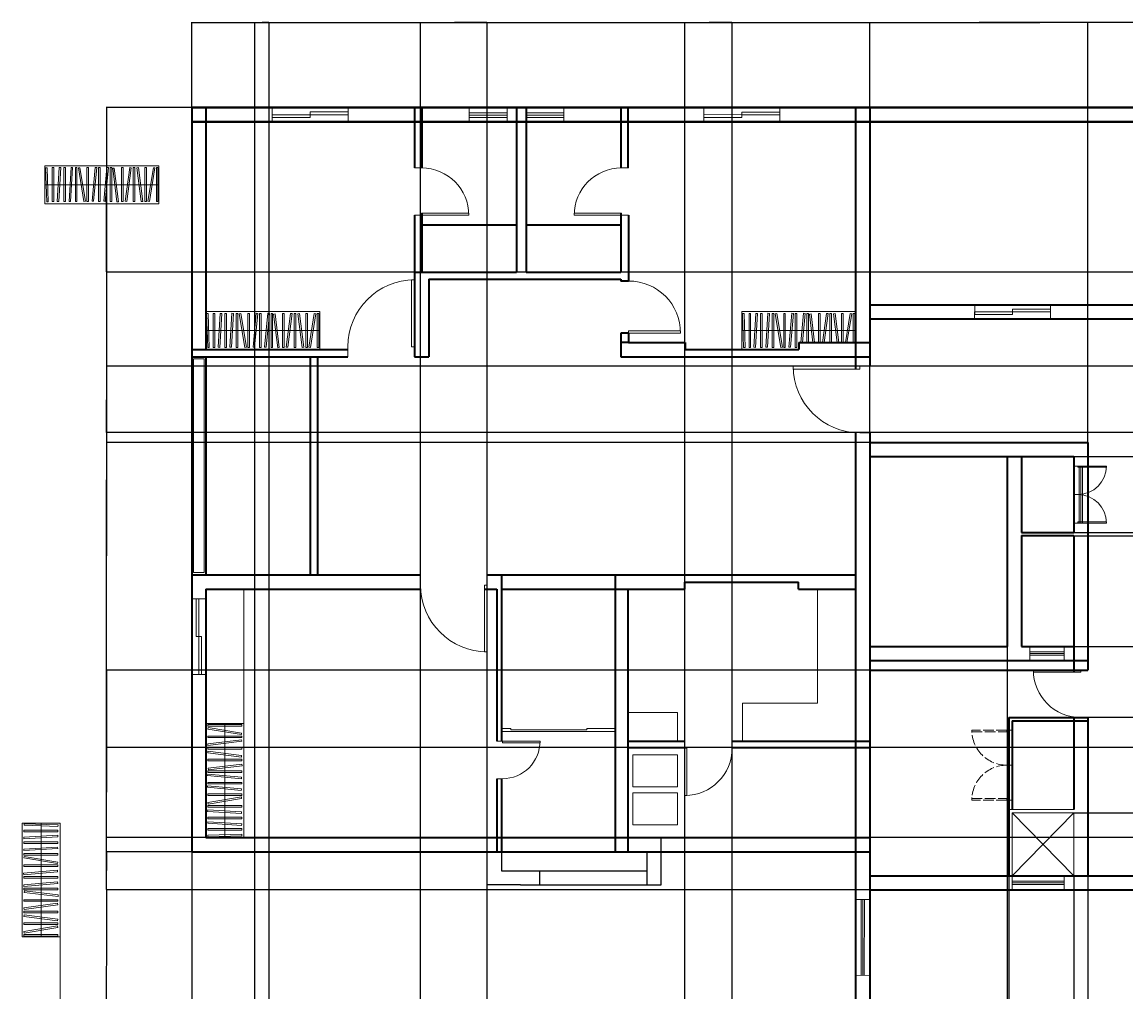
# Model space of a CAD drawing. Units: inches. Extents: x 531915 to 533151, y 849859 to 851471.
# Tile 5 of 7: x 531915 to 532614, y 850858 to 851471. Entities that reach past the tile are written whole.
import ezdxf

# ---------------------------------------------------------------- set-up
doc = ezdxf.new("R2010")
doc.units = ezdxf.units.IN
doc.linetypes.add('ACAD_ISO02W100', pattern=[15, 12, -3])
for name, color, linetype, lineweight in [('A-ANNO-DIMS', 2, 'Continuous', 18), ('A-DOOR', 3, 'Continuous', 18), ('A-DOOR-HIDN', 3, 'ACAD_ISO02W100', 18), ('A-FLOR-CASE', 9, 'Continuous', 18), ('A-FLOR-FIXT', 8, 'Continuous', 18), ('A-FLOR-HRAL', 4, 'Continuous', 20), ('A-FLOR-SHFT', 9, 'Continuous', 18), ('A-FLOR-SLAB', 7, 'Continuous', 25), ('A-FURN', 8, 'Continuous', 13), ('A-GLAZ', 4, 'Continuous', 18), ('A-WALL', 7, 'Continuous', 35)]:
    doc.layers.add(name, color=color, linetype=linetype, lineweight=lineweight)
doc.styles.get("Standard").update_dxf_attribs({"font": 'arial.ttf'})
doc.dimstyles.get("Standard").update_dxf_attribs({"dimtxt": 0.18, "dimasz": 0.18, "dimexe": 0.18, "dimexo": 0.0625, "dimgap": 0.09, "dimtad": 0, "dimtih": 1, "dimtoh": 1, "dimdec": 4, "dimzin": 0, "dimdsep": 46, "dimtxsty": 'Standard', "dimcen": 0.09, "dimadec": 0, "dimazin": 0, "dimtfac": 1, "dimtdec": 4, "dimtofl": 0, "dimtmove": 0, "dimatfit": 3, "dimfxl": 1, "dimtolj": 1, "dimtzin": 0, "dimarcsym": 0})

# ---------------------------------------------------------------- blocks, each defined once
blk = doc.blocks.new('*U2')
for p, q in [((0, 0), (0, -6)), ((40, 0), (40, -6))]:
    blk.add_line(p, q)
blk.add_lwpolyline([(0, 0), (0, 40), (1.75, 40), (1.75, 0)], close=True)
blk.add_arc((0, 0), 40, 0, 90)
blk = doc.blocks.new('WARDROBE-72')
blk.add_line((12, 0), (12, 72))
for points in [[(24, 0), (24, 72), (0, 72), (0, 0)], [(1.15, 70.47), (1.15, 71.48), (22.64, 71.48), (22.64, 70.47)], [(1.15, 63.15), (1.15, 64.16), (22.64, 64.16), (22.64, 63.15)], [(1.21, 68.56), (1.37, 69.55), (22.58, 66.07), (22.41, 65.07)], [(1.15, 55.83), (1.15, 56.84), (22.64, 56.84), (22.64, 55.83)], [(1.3, 58.13), (1.17, 59.13), (22.48, 61.86), (22.61, 60.86)], [(1.11, 53.59), (1.24, 54.59), (22.54, 51.79), (22.41, 50.79)], [(1.15, 48.51), (1.15, 49.52), (22.64, 49.52), (22.64, 48.51)], [(1.15, 41.19), (1.15, 42.2), (22.64, 42.2), (22.64, 41.19)], [(1.55, 42.84), (1.42, 43.84), (22.76, 46.42), (22.88, 45.42)], [(1.04, 39.13), (1.13, 40.14), (22.52, 38.16), (22.43, 37.15)], [(0.98, 31.76), (1.07, 32.76), (22.47, 30.78), (22.37, 29.78)], [(1.15, 33.87), (1.15, 34.88), (22.64, 34.88), (22.64, 33.87)], [(1.15, 26.55), (1.15, 27.56), (22.64, 27.56), (22.64, 26.55)], [(1.38, 21.1), (1.21, 22.1), (22.4, 25.68), (22.57, 24.68)], [(1.05, 16.46), (1.11, 17.47), (22.56, 16.21), (22.5, 15.2)], [(1.15, 19.23), (1.15, 20.24), (22.64, 20.24), (22.64, 19.23)], [(1.11, 8.97), (1.17, 9.98), (22.62, 8.71), (22.56, 7.7)], [(1.15, 11.91), (1.15, 12.92), (22.64, 12.92), (22.64, 11.91)], [(1.15, 4.59), (1.15, 5.6), (22.64, 5.6), (22.64, 4.59)], [(1.25, 0.42), (1.22, 1.43), (22.7, 2.11), (22.73, 1.1)]]:
    blk.add_lwpolyline(points, close=True)
blk = doc.blocks.new('WARDROBE-72-RECESSED')
blk.add_line((0, 12), (72, 12))
for points in [[(72, 0), (72, 24), (0, 24), (0, 0), (36.16, 0)], [(37.42, 4.5), (39.13, 22.96), (40.14, 22.87), (38.44, 4.5)], [(41.19, 4.5), (41.19, 22.85), (42.2, 22.85), (42.2, 4.5)], [(45.01, 4.5), (42.84, 22.45), (43.84, 22.58), (46.03, 4.5)], [(48.51, 4.5), (48.51, 22.85), (49.52, 22.85), (49.52, 4.5)], [(51.17, 4.5), (53.59, 22.89), (54.59, 22.76), (52.19, 4.5)], [(55.83, 4.5), (55.83, 22.85), (56.84, 22.85), (56.84, 4.5)], [(60.46, 4.5), (58.13, 22.7), (59.13, 22.83), (61.48, 4.5)], [(63.15, 4.5), (63.15, 22.85), (64.16, 22.85), (64.16, 4.5)], [(65.55, 4.5), (68.56, 22.79), (69.55, 22.63), (66.57, 4.5)], [(70.47, 4.5), (70.47, 22.85), (71.48, 22.85), (71.48, 4.5)]]:
    blk.add_lwpolyline(points)
for points in [[(0.42, 22.75), (1.43, 22.78), (2.11, 1.3), (1.1, 1.27)], [(4.59, 22.85), (5.6, 22.85), (5.6, 1.36), (4.59, 1.36)], [(8.97, 22.89), (9.98, 22.83), (8.71, 1.38), (7.7, 1.44)], [(11.91, 22.85), (12.92, 22.85), (12.92, 1.36), (11.91, 1.36)], [(16.46, 22.95), (17.47, 22.89), (16.21, 1.44), (15.2, 1.5)], [(19.23, 22.85), (20.24, 22.85), (20.24, 1.36), (19.23, 1.36)], [(21.1, 22.62), (22.1, 22.79), (25.68, 1.6), (24.68, 1.43)], [(26.55, 22.85), (27.56, 22.85), (27.56, 1.36), (26.55, 1.36)], [(31.76, 23.02), (32.76, 22.93), (30.78, 1.53), (29.78, 1.63)], [(33.87, 22.85), (34.88, 22.85), (34.88, 1.36), (33.87, 1.36)]]:
    blk.add_lwpolyline(points, close=True)
blk = doc.blocks.new('WINDOW-SLIDING-48')
for p, q in [((0, 9), (0, 0)), ((48, 9), (48, 0)), ((0, 4.5), (48, 4.5))]:
    blk.add_line(p, q)
for points in [[(24, 4.5), (0, 4.5), (0, 2.84), (24, 2.84)], [(24, 4.5), (48, 4.5), (48, 6.29), (24, 6.29)]]:
    blk.add_lwpolyline(points, close=True)
blk = doc.blocks.new('WINDOW-VENT-24')
blk.add_line((0, 1.44), (24, 1.44))
blk.add_lwpolyline([(0, 2.89), (24, 2.89), (24, 0), (0, 0)], close=True)
blk = doc.blocks.new('UTILITY-FIXTURES-PAIR')
for points in [[(0, 24.11), (28.12, 24.11), (28.12, 44.31), (0, 44.31)], [(0, 0), (28.12, 0), (28.12, 20.2), (0, 20.2)]]:
    blk.add_lwpolyline(points, close=True)
blk = doc.blocks.new('SLIDING-PANEL-72')
for p, q in [((0, 2), (6, 2)), ((6, 2), (6, 1)), ((6, 1), (54, 1)), ((54, 2), (72, 2)), ((54, 2), (54, 1)), ((0, 0), (72, 0))]:
    blk.add_line(p, q)
blk = doc.blocks.new('COUNTER-L-RETURN')
for p, q in [((47.51, 96), (47.51, 24)), ((0, 24), (47.51, 24)), ((0, 24), (0, 0))]:
    blk.add_line(p, q)
blk = doc.blocks.new('COUNTER-END-RETURN')
for p in [(0, 18), (31.29, 0)]:
    blk.add_line(p, (31.29, 18))
blk = doc.blocks.new('*D37')
at = {"layer": 'A-ANNO-DIMS', "color": 0, "lineweight": -2, "transparency": 16777216}
for p, q in [((532022.8, 851416.94), (532022.8, 851470.96)), ((532022.98, 851470.78), (532559.45, 851470.78)), ((533096.62, 851470.78), (532560.15, 851470.78)), ((533096.8, 851416.94), (533096.8, 851470.96))]:
    blk.add_line(p, q, dxfattribs=at)
at = {"layer": 'A-ANNO-DIMS', "color": 0, "transparency": 16777216}
for points in [[(532022.98, 851470.81), (532022.98, 851470.75), (532022.8, 851470.78)], [(533096.62, 851470.81), (533096.62, 851470.75), (533096.8, 851470.78)]]:
    blk.add_solid(points, dxfattribs=at)
at = {"layer": 'Defpoints', "color": 0, "transparency": 16777216}
for p in [(533096.8, 851470.78), (532022.8, 851416.87), (533096.8, 851416.87)]:
    blk.add_point(p, dxfattribs=at)
at = {"layer": 'A-ANNO-DIMS', "color": 0, "transparency": 16777216, "insert": (532559.8, 851470.78), "char_height": 0.18, "attachment_point": 5}
blk.add_mtext('\\A1;1074', dxfattribs=at)
blk = doc.blocks.new('*D39')
at = {"layer": 'A-ANNO-DIMS', "color": 0, "lineweight": -2, "transparency": 16777216}
for p, q in [((532022.74, 851416.87), (531968.71, 851416.87)), ((531968.89, 851416.69), (531968.89, 851181.81)), ((531968.89, 850946.55), (531968.89, 851181.44)), ((532022.74, 850946.37), (531968.71, 850946.37))]:
    blk.add_line(p, q, dxfattribs=at)
at = {"layer": 'A-ANNO-DIMS', "color": 0, "transparency": 16777216}
for points in [[(531968.86, 851416.69), (531968.92, 851416.69), (531968.89, 851416.87)], [(531968.86, 850946.55), (531968.92, 850946.55), (531968.89, 850946.37)]]:
    blk.add_solid(points, dxfattribs=at)
at = {"layer": 'Defpoints', "color": 0, "transparency": 16777216}
for p in [(532022.8, 851416.87), (531968.89, 850946.37), (532022.8, 850946.37)]:
    blk.add_point(p, dxfattribs=at)
at = {"layer": 'A-ANNO-DIMS', "color": 0, "transparency": 16777216, "insert": (531968.89, 851181.62), "char_height": 0.18, "attachment_point": 5}
blk.add_mtext('\\A1;470.5', dxfattribs=at)
blk = doc.blocks.new('*D40')
at = {"layer": 'A-ANNO-DIMS', "color": 0, "lineweight": -2, "transparency": 16777216}
for p, q in [((532022.74, 850946.37), (531968.71, 850946.37)), ((531968.89, 850946.19), (531968.89, 850934.48)), ((531968.89, 850922.41), (531968.89, 850934.12)), ((532451.74, 850922.23), (531968.71, 850922.23))]:
    blk.add_line(p, q, dxfattribs=at)
at = {"layer": 'A-ANNO-DIMS', "color": 0, "transparency": 16777216}
for points in [[(531968.86, 850946.19), (531968.92, 850946.19), (531968.89, 850946.37)], [(531968.86, 850922.41), (531968.92, 850922.41), (531968.89, 850922.23)]]:
    blk.add_solid(points, dxfattribs=at)
at = {"layer": 'Defpoints', "color": 0, "transparency": 16777216}
for p in [(532022.8, 850946.37), (531968.89, 850922.23), (532451.8, 850922.23)]:
    blk.add_point(p, dxfattribs=at)
at = {"layer": 'A-ANNO-DIMS', "color": 0, "transparency": 16777216, "insert": (531968.89, 850934.3), "char_height": 0.18, "attachment_point": 5}
blk.add_mtext('\\A1;24.14', dxfattribs=at)
blk = doc.blocks.new('*D41')
at = {"layer": 'A-ANNO-DIMS', "color": 0, "lineweight": -2, "transparency": 16777216}
for p, q in [((532451.74, 850922.23), (531968.71, 850922.23)), ((531968.89, 850922.05), (531968.89, 850874.49)), ((531968.89, 850826.55), (531968.89, 850874.12)), ((532062.74, 850826.37), (531968.71, 850826.37))]:
    blk.add_line(p, q, dxfattribs=at)
at = {"layer": 'A-ANNO-DIMS', "color": 0, "transparency": 16777216}
for points in [[(531968.86, 850922.05), (531968.92, 850922.05), (531968.89, 850922.23)], [(531968.86, 850826.55), (531968.92, 850826.55), (531968.89, 850826.37)]]:
    blk.add_solid(points, dxfattribs=at)
at = {"layer": 'Defpoints', "color": 0, "transparency": 16777216}
for p in [(532451.8, 850922.23), (531968.89, 850826.37), (532062.8, 850826.37)]:
    blk.add_point(p, dxfattribs=at)
at = {"layer": 'A-ANNO-DIMS', "color": 0, "transparency": 16777216, "insert": (531968.89, 850874.3), "char_height": 0.18, "attachment_point": 5}
blk.add_mtext('\\A1;95.86', dxfattribs=at)
blk = doc.blocks.new('*D46')
at = {"layer": 'A-ANNO-DIMS', "color": 0, "lineweight": -2, "transparency": 16777216}
for p, q in [((532022.8, 850946.31), (532022.8, 850315.34)), ((532062.8, 850826.31), (532062.8, 850315.34)), ((532022.98, 850315.52), (532042.58, 850315.52)), ((532062.62, 850315.52), (532043.03, 850315.52))]:
    blk.add_line(p, q, dxfattribs=at)
at = {"layer": 'A-ANNO-DIMS', "color": 0, "transparency": 16777216}
for points in [[(532022.98, 850315.55), (532022.98, 850315.49), (532022.8, 850315.52)], [(532062.62, 850315.55), (532062.62, 850315.49), (532062.8, 850315.52)]]:
    blk.add_solid(points, dxfattribs=at)
at = {"layer": 'Defpoints', "color": 0, "transparency": 16777216}
for p in [(532022.8, 850946.37), (532062.8, 850826.37), (532062.8, 850315.52)]:
    blk.add_point(p, dxfattribs=at)
at = {"layer": 'A-ANNO-DIMS', "color": 0, "transparency": 16777216, "insert": (532042.8, 850315.52), "char_height": 0.18, "attachment_point": 5}
blk.add_mtext('\\A1;40', dxfattribs=at)
blk = doc.blocks.new('*D59')
at = {"layer": 'A-ANNO-DIMS', "color": 0, "lineweight": -2, "transparency": 16777216}
for p, q in [((533087.74, 851012.37), (531968.71, 851012.37)), ((531968.89, 851012.19), (531968.89, 850984.06)), ((531968.89, 850955.55), (531968.89, 850983.69)), ((533087.74, 850955.37), (531968.71, 850955.37))]:
    blk.add_line(p, q, dxfattribs=at)
at = {"layer": 'A-ANNO-DIMS', "color": 0, "transparency": 16777216}
for points in [[(531968.86, 851012.19), (531968.92, 851012.19), (531968.89, 851012.37)], [(531968.86, 850955.55), (531968.92, 850955.55), (531968.89, 850955.37)]]:
    blk.add_solid(points, dxfattribs=at)
at = {"layer": 'Defpoints', "color": 0, "transparency": 16777216}
for p in [(533087.8, 851012.37), (531968.89, 850955.37), (533087.8, 850955.37)]:
    blk.add_point(p, dxfattribs=at)
at = {"layer": 'A-ANNO-DIMS', "color": 0, "transparency": 16777216, "insert": (531968.89, 850983.87), "char_height": 0.18, "attachment_point": 5}
blk.add_mtext('\\A1;57', dxfattribs=at)
blk = doc.blocks.new('*D68')
at = {"layer": 'A-ANNO-DIMS', "color": 0, "lineweight": -2, "transparency": 16777216}
for p, q in [((532451.74, 851205.23), (531968.71, 851205.23)), ((531968.89, 851205.05), (531968.89, 851133.41)), ((531968.89, 851061.41), (531968.89, 851133.05)), ((532451.74, 851061.23), (531968.71, 851061.23))]:
    blk.add_line(p, q, dxfattribs=at)
at = {"layer": 'A-ANNO-DIMS', "color": 0, "transparency": 16777216}
for points in [[(531968.86, 851205.05), (531968.92, 851205.05), (531968.89, 851205.23)], [(531968.86, 851061.41), (531968.92, 851061.41), (531968.89, 851061.23)]]:
    blk.add_solid(points, dxfattribs=at)
at = {"layer": 'Defpoints', "color": 0, "transparency": 16777216}
for p in [(532451.8, 851205.23), (531968.89, 851061.23), (532451.8, 851061.23)]:
    blk.add_point(p, dxfattribs=at)
at = {"layer": 'A-ANNO-DIMS', "color": 0, "transparency": 16777216, "insert": (531968.89, 851133.23), "char_height": 0.18, "attachment_point": 5}
blk.add_mtext('\\A1;144', dxfattribs=at)
blk = doc.blocks.new('*D69')
at = {"layer": 'A-ANNO-DIMS', "color": 0, "lineweight": -2, "transparency": 16777216}
for p, q in [((532451.74, 851061.23), (531968.71, 851061.23)), ((531968.89, 851061.05), (531968.89, 850991.92)), ((531968.89, 850922.41), (531968.89, 850991.55)), ((532451.74, 850922.23), (531968.71, 850922.23))]:
    blk.add_line(p, q, dxfattribs=at)
at = {"layer": 'A-ANNO-DIMS', "color": 0, "transparency": 16777216}
for points in [[(531968.86, 851061.05), (531968.92, 851061.05), (531968.89, 851061.23)], [(531968.86, 850922.41), (531968.92, 850922.41), (531968.89, 850922.23)]]:
    blk.add_solid(points, dxfattribs=at)
at = {"layer": 'Defpoints', "color": 0, "transparency": 16777216}
for p in [(532451.8, 851061.23), (531968.89, 850922.23), (532451.8, 850922.23)]:
    blk.add_point(p, dxfattribs=at)
at = {"layer": 'A-ANNO-DIMS', "color": 0, "transparency": 16777216, "insert": (531968.89, 850991.73), "char_height": 0.18, "attachment_point": 5}
blk.add_mtext('\\A1;139', dxfattribs=at)
blk = doc.blocks.new('*D70')
at = {"layer": 'A-ANNO-DIMS', "color": 0, "lineweight": -2, "transparency": 16777216}
for p, q in [((532451.8, 851205.3), (532451.8, 851470.96)), ((532451.98, 851470.78), (532520.52, 851470.78)), ((532589.62, 851470.78), (532521.09, 851470.78)), ((532589.8, 851205.3), (532589.8, 851470.96))]:
    blk.add_line(p, q, dxfattribs=at)
at = {"layer": 'A-ANNO-DIMS', "color": 0, "transparency": 16777216}
for points in [[(532451.98, 851470.81), (532451.98, 851470.75), (532451.8, 851470.78)], [(532589.62, 851470.81), (532589.62, 851470.75), (532589.8, 851470.78)]]:
    blk.add_solid(points, dxfattribs=at)
at = {"layer": 'Defpoints', "color": 0, "transparency": 16777216}
for p in [(532589.8, 851470.78), (532451.8, 851205.23), (532589.8, 851205.23)]:
    blk.add_point(p, dxfattribs=at)
at = {"layer": 'A-ANNO-DIMS', "color": 0, "transparency": 16777216, "insert": (532520.8, 851470.78), "char_height": 0.18, "attachment_point": 5}
blk.add_mtext('\\A1;138', dxfattribs=at)
blk = doc.blocks.new('*D71')
at = {"layer": 'A-ANNO-DIMS', "color": 0, "lineweight": -2, "transparency": 16777216}
for p, q in [((532589.8, 850931.17), (532589.8, 850315.34)), ((532667.8, 850931.17), (532667.8, 850315.34)), ((532589.98, 850315.52), (532628.59, 850315.52)), ((532667.62, 850315.52), (532629.02, 850315.52))]:
    blk.add_line(p, q, dxfattribs=at)
at = {"layer": 'A-ANNO-DIMS', "color": 0, "transparency": 16777216}
for points in [[(532589.98, 850315.55), (532589.98, 850315.49), (532589.8, 850315.52)], [(532667.62, 850315.55), (532667.62, 850315.49), (532667.8, 850315.52)]]:
    blk.add_solid(points, dxfattribs=at)
at = {"layer": 'Defpoints', "color": 0, "transparency": 16777216}
for p in [(532589.8, 850931.23), (532667.8, 850931.23), (532667.8, 850315.52)]:
    blk.add_point(p, dxfattribs=at)
at = {"layer": 'A-ANNO-DIMS', "color": 0, "transparency": 16777216, "insert": (532628.8, 850315.52), "char_height": 0.18, "attachment_point": 5}
blk.add_mtext('\\A1;78', dxfattribs=at)
blk = doc.blocks.new('*D72')
at = {"layer": 'A-ANNO-DIMS', "color": 0, "lineweight": -2, "transparency": 16777216}
for p, q in [((532451.8, 850931.17), (532451.8, 850315.34)), ((532539.8, 850931.17), (532539.8, 850315.34)), ((532451.98, 850315.52), (532495.59, 850315.52)), ((532539.62, 850315.52), (532496.02, 850315.52))]:
    blk.add_line(p, q, dxfattribs=at)
at = {"layer": 'A-ANNO-DIMS', "color": 0, "transparency": 16777216}
for points in [[(532451.98, 850315.55), (532451.98, 850315.49), (532451.8, 850315.52)], [(532539.62, 850315.55), (532539.62, 850315.49), (532539.8, 850315.52)]]:
    blk.add_solid(points, dxfattribs=at)
at = {"layer": 'Defpoints', "color": 0, "transparency": 16777216}
for p in [(532451.8, 850931.23), (532539.8, 850931.23), (532539.8, 850315.52)]:
    blk.add_point(p, dxfattribs=at)
at = {"layer": 'A-ANNO-DIMS', "color": 0, "transparency": 16777216, "insert": (532495.8, 850315.52), "char_height": 0.18, "attachment_point": 5}
blk.add_mtext('\\A1;88', dxfattribs=at)
blk = doc.blocks.new('*D73')
at = {"layer": 'A-ANNO-DIMS', "color": 0, "lineweight": -2, "transparency": 16777216}
for p, q in [((532539.8, 850931.17), (532539.8, 850315.34)), ((532580.8, 850931.17), (532580.8, 850315.34)), ((532539.98, 850315.52), (532560.1, 850315.52)), ((532580.62, 850315.52), (532560.51, 850315.52))]:
    blk.add_line(p, q, dxfattribs=at)
at = {"layer": 'A-ANNO-DIMS', "color": 0, "transparency": 16777216}
for points in [[(532539.98, 850315.55), (532539.98, 850315.49), (532539.8, 850315.52)], [(532580.62, 850315.55), (532580.62, 850315.49), (532580.8, 850315.52)]]:
    blk.add_solid(points, dxfattribs=at)
at = {"layer": 'Defpoints', "color": 0, "transparency": 16777216}
for p in [(532539.8, 850931.23), (532580.8, 850931.23), (532580.8, 850315.52)]:
    blk.add_point(p, dxfattribs=at)
at = {"layer": 'A-ANNO-DIMS', "color": 0, "transparency": 16777216, "insert": (532560.3, 850315.52), "char_height": 0.18, "attachment_point": 5}
blk.add_mtext('\\A1;41', dxfattribs=at)
blk = doc.blocks.new('*D74')
at = {"layer": 'A-ANNO-DIMS', "color": 0, "lineweight": -2, "transparency": 16777216}
for p, q in [((532580.87, 850971.01), (533150.9, 850971.01)), ((533150.72, 850970.83), (533150.72, 850951.31)), ((533150.72, 850931.41), (533150.72, 850950.94)), ((532580.87, 850931.23), (533150.9, 850931.23))]:
    blk.add_line(p, q, dxfattribs=at)
at = {"layer": 'A-ANNO-DIMS', "color": 0, "transparency": 16777216}
for points in [[(533150.69, 850970.83), (533150.75, 850970.83), (533150.72, 850971.01)], [(533150.69, 850931.41), (533150.75, 850931.41), (533150.72, 850931.23)]]:
    blk.add_solid(points, dxfattribs=at)
at = {"layer": 'Defpoints', "color": 0, "transparency": 16777216}
for p in [(532580.8, 850971.01), (533150.72, 850971.01), (532580.8, 850931.23)]:
    blk.add_point(p, dxfattribs=at)
at = {"layer": 'A-ANNO-DIMS', "color": 0, "transparency": 16777216, "insert": (533150.72, 850951.12), "char_height": 0.18, "attachment_point": 5}
blk.add_mtext('\\A1;39.78', dxfattribs=at)
blk = doc.blocks.new('*D75')
at = {"layer": 'A-ANNO-DIMS', "color": 0, "lineweight": -2, "transparency": 16777216}
for p, q in [((532580.87, 851031.56), (533150.9, 851031.56)), ((533150.72, 851031.38), (533150.72, 851001.47)), ((533150.72, 850971.19), (533150.72, 851001.11)), ((532580.87, 850971.01), (533150.9, 850971.01))]:
    blk.add_line(p, q, dxfattribs=at)
at = {"layer": 'A-ANNO-DIMS', "color": 0, "transparency": 16777216}
for points in [[(533150.69, 851031.38), (533150.75, 851031.38), (533150.72, 851031.56)], [(533150.69, 850971.19), (533150.75, 850971.19), (533150.72, 850971.01)]]:
    blk.add_solid(points, dxfattribs=at)
at = {"layer": 'Defpoints', "color": 0, "transparency": 16777216}
for p in [(532580.8, 851031.56), (533150.72, 851031.56), (532580.8, 850971.01)]:
    blk.add_point(p, dxfattribs=at)
at = {"layer": 'A-ANNO-DIMS', "color": 0, "transparency": 16777216, "insert": (533150.72, 851001.29), "char_height": 0.18, "attachment_point": 5}
blk.add_mtext('\\A1;60.55', dxfattribs=at)
blk = doc.blocks.new('*D76')
at = {"layer": 'A-ANNO-DIMS', "color": 0, "lineweight": -2, "transparency": 16777216}
for p, q in [((532820.74, 851416.87), (531968.71, 851416.87)), ((531968.89, 851416.69), (531968.89, 851365.03)), ((531968.89, 851313), (531968.89, 851364.67)), ((532825.24, 851312.82), (531968.71, 851312.82))]:
    blk.add_line(p, q, dxfattribs=at)
at = {"layer": 'A-ANNO-DIMS', "color": 0, "transparency": 16777216}
for points in [[(531968.86, 851416.69), (531968.92, 851416.69), (531968.89, 851416.87)], [(531968.86, 851313), (531968.92, 851313), (531968.89, 851312.82)]]:
    blk.add_solid(points, dxfattribs=at)
at = {"layer": 'Defpoints', "color": 0, "transparency": 16777216}
for p in [(532820.8, 851416.87), (531968.89, 851312.82), (532825.3, 851312.82)]:
    blk.add_point(p, dxfattribs=at)
at = {"layer": 'A-ANNO-DIMS', "color": 0, "transparency": 16777216, "insert": (531968.89, 851364.85), "char_height": 0.18, "attachment_point": 5}
blk.add_mtext('\\A1;104.05', dxfattribs=at)
blk = doc.blocks.new('*D78')
at = {"layer": 'A-ANNO-DIMS', "color": 0, "lineweight": -2, "transparency": 16777216}
for p, q in [((532451.8, 851196.17), (532451.8, 850315.34)), ((532538.8, 851196.17), (532538.8, 850315.34)), ((532451.98, 850315.52), (532495.09, 850315.52)), ((532538.62, 850315.52), (532495.52, 850315.52))]:
    blk.add_line(p, q, dxfattribs=at)
at = {"layer": 'A-ANNO-DIMS', "color": 0, "transparency": 16777216}
for points in [[(532451.98, 850315.55), (532451.98, 850315.49), (532451.8, 850315.52)], [(532538.62, 850315.55), (532538.62, 850315.49), (532538.8, 850315.52)]]:
    blk.add_solid(points, dxfattribs=at)
at = {"layer": 'Defpoints', "color": 0, "transparency": 16777216}
for p in [(532451.8, 851196.23), (532538.8, 851196.23), (532538.8, 850315.52)]:
    blk.add_point(p, dxfattribs=at)
at = {"layer": 'A-ANNO-DIMS', "color": 0, "transparency": 16777216, "insert": (532495.3, 850315.52), "char_height": 0.18, "attachment_point": 5}
blk.add_mtext('\\A1;87', dxfattribs=at)
blk = doc.blocks.new('*D79')
at = {"layer": 'A-ANNO-DIMS', "color": 0, "lineweight": -2, "transparency": 16777216}
for p, q in [((532580.87, 851196.23), (533150.9, 851196.23)), ((533150.72, 851196.05), (533150.72, 851172.42)), ((533150.72, 851148.41), (533150.72, 851172.05)), ((532580.87, 851148.23), (533150.9, 851148.23))]:
    blk.add_line(p, q, dxfattribs=at)
at = {"layer": 'A-ANNO-DIMS', "color": 0, "transparency": 16777216}
for points in [[(533150.69, 851196.05), (533150.75, 851196.05), (533150.72, 851196.23)], [(533150.69, 851148.41), (533150.75, 851148.41), (533150.72, 851148.23)]]:
    blk.add_solid(points, dxfattribs=at)
at = {"layer": 'Defpoints', "color": 0, "transparency": 16777216}
for p in [(532580.8, 851196.23), (532580.8, 851148.23), (533150.72, 851148.23)]:
    blk.add_point(p, dxfattribs=at)
at = {"layer": 'A-ANNO-DIMS', "color": 0, "transparency": 16777216, "insert": (533150.72, 851172.23), "char_height": 0.18, "attachment_point": 5}
blk.add_mtext('\\A1;48', dxfattribs=at)
blk = doc.blocks.new('*D80')
at = {"layer": 'A-ANNO-DIMS', "color": 0, "lineweight": -2, "transparency": 16777216}
for p, q in [((532580.87, 851146.23), (533150.9, 851146.23)), ((533150.72, 851146.05), (533150.72, 851111.42)), ((533150.72, 851076.41), (533150.72, 851111.05)), ((532580.87, 851076.23), (533150.9, 851076.23))]:
    blk.add_line(p, q, dxfattribs=at)
at = {"layer": 'A-ANNO-DIMS', "color": 0, "transparency": 16777216}
for points in [[(533150.69, 851146.05), (533150.75, 851146.05), (533150.72, 851146.23)], [(533150.69, 851076.41), (533150.75, 851076.41), (533150.72, 851076.23)]]:
    blk.add_solid(points, dxfattribs=at)
at = {"layer": 'Defpoints', "color": 0, "transparency": 16777216}
for p in [(532580.8, 851146.23), (532580.8, 851076.23), (533150.72, 851076.23)]:
    blk.add_point(p, dxfattribs=at)
at = {"layer": 'A-ANNO-DIMS', "color": 0, "transparency": 16777216, "insert": (533150.72, 851111.23), "char_height": 0.18, "attachment_point": 5}
blk.add_mtext('\\A1;70', dxfattribs=at)
blk = doc.blocks.new('*D81')
at = {"layer": 'A-ANNO-DIMS', "color": 0, "lineweight": -2, "transparency": 16777216}
for p, q in [((532062.8, 850826.44), (532062.8, 851470.96)), ((532062.98, 851470.78), (532067.16, 851470.78)), ((532071.62, 851470.78), (532067.45, 851470.78)), ((532071.8, 850817.44), (532071.8, 851470.96))]:
    blk.add_line(p, q, dxfattribs=at)
at = {"layer": 'A-ANNO-DIMS', "color": 0, "transparency": 16777216}
for points in [[(532062.98, 851470.81), (532062.98, 851470.75), (532062.8, 851470.78)], [(532071.62, 851470.81), (532071.62, 851470.75), (532071.8, 851470.78)]]:
    blk.add_solid(points, dxfattribs=at)
at = {"layer": 'Defpoints', "color": 0, "transparency": 16777216}
for p in [(532071.8, 851470.78), (532062.8, 850826.37), (532071.8, 850817.37)]:
    blk.add_point(p, dxfattribs=at)
at = {"layer": 'A-ANNO-DIMS', "color": 0, "transparency": 16777216, "insert": (532067.3, 851470.78), "char_height": 0.18, "attachment_point": 5}
blk.add_mtext('\\A1;9', dxfattribs=at)
blk = doc.blocks.new('*D83')
at = {"layer": 'A-ANNO-DIMS', "color": 0, "lineweight": -2, "transparency": 16777216}
for p, q in [((532667.74, 851253.37), (531968.71, 851253.37)), ((531968.89, 851253.19), (531968.89, 851232.55)), ((531968.89, 851211.55), (531968.89, 851232.19)), ((532667.74, 851211.37), (531968.71, 851211.37))]:
    blk.add_line(p, q, dxfattribs=at)
at = {"layer": 'A-ANNO-DIMS', "color": 0, "transparency": 16777216}
for points in [[(531968.86, 851253.19), (531968.92, 851253.19), (531968.89, 851253.37)], [(531968.86, 851211.55), (531968.92, 851211.55), (531968.89, 851211.37)]]:
    blk.add_solid(points, dxfattribs=at)
at = {"layer": 'Defpoints', "color": 0, "transparency": 16777216}
for p in [(531968.89, 851253.37), (532667.8, 851253.37), (532667.8, 851211.37)]:
    blk.add_point(p, dxfattribs=at)
at = {"layer": 'A-ANNO-DIMS', "color": 0, "transparency": 16777216, "insert": (531968.89, 851232.37), "char_height": 0.18, "attachment_point": 5}
blk.add_mtext('\\A1;42', dxfattribs=at)
blk = doc.blocks.new('*D85')
at = {"layer": 'A-ANNO-DIMS', "color": 0, "lineweight": -2, "transparency": 16777216}
for p, q in [((532334.8, 850439.44), (532334.8, 851470.96)), ((532334.98, 851470.78), (532349.32, 851470.78)), ((532364.58, 851470.78), (532350.25, 851470.78)), ((532364.76, 850439.44), (532364.76, 851470.96))]:
    blk.add_line(p, q, dxfattribs=at)
at = {"layer": 'A-ANNO-DIMS', "color": 0, "transparency": 16777216}
for points in [[(532334.98, 851470.81), (532334.98, 851470.75), (532334.8, 851470.78)], [(532364.58, 851470.81), (532364.58, 851470.75), (532364.76, 851470.78)]]:
    blk.add_solid(points, dxfattribs=at)
at = {"layer": 'Defpoints', "color": 0, "transparency": 16777216}
for p in [(532364.76, 851470.78), (532334.8, 850439.37), (532364.76, 850439.37)]:
    blk.add_point(p, dxfattribs=at)
at = {"layer": 'A-ANNO-DIMS', "color": 0, "transparency": 16777216, "insert": (532349.78, 851470.78), "char_height": 0.18, "attachment_point": 5}
blk.add_mtext('\\A1;29.954', dxfattribs=at)
blk = doc.blocks.new('*D86')
at = {"layer": 'A-ANNO-DIMS', "color": 0, "lineweight": -2, "transparency": 16777216}
for p, q in [((532167.55, 850544.44), (532167.55, 851470.96)), ((532167.73, 851470.78), (532188.28, 851470.78)), ((532209.62, 851470.78), (532189.08, 851470.78)), ((532209.8, 850544.44), (532209.8, 851470.96))]:
    blk.add_line(p, q, dxfattribs=at)
at = {"layer": 'A-ANNO-DIMS', "color": 0, "transparency": 16777216}
for points in [[(532167.73, 851470.81), (532167.73, 851470.75), (532167.55, 851470.78)], [(532209.62, 851470.81), (532209.62, 851470.75), (532209.8, 851470.78)]]:
    blk.add_solid(points, dxfattribs=at)
at = {"layer": 'Defpoints', "color": 0, "transparency": 16777216}
for p in [(532209.8, 851470.78), (532167.55, 850544.37), (532209.8, 850544.37)]:
    blk.add_point(p, dxfattribs=at)
at = {"layer": 'A-ANNO-DIMS', "color": 0, "transparency": 16777216, "insert": (532188.68, 851470.78), "char_height": 0.18, "attachment_point": 5}
blk.add_mtext('\\A1;42.25', dxfattribs=at)

msp = doc.modelspace()

# ---------------------------------------------------------------- linework, layer by layer
at = {"layer": 'A-DOOR'}
for p, q in [((532580.8048, 851190.2344), (532589.8048, 851190.2344)), ((532584.3048, 851190.2344), (532584.3048, 851154.2344)), ((532585.3048, 851190.2344), (532585.3048, 851154.2344)), ((532586.3048, 851190.2344), (532586.3048, 851154.2344)), ((532580.8048, 851154.2344), (532589.8048, 851154.2344))]:
    msp.add_line(p, q, dxfattribs=at)
at = {"layer": 'A-FLOR-CASE'}
msp.add_line((532442.8048, 851112.374), (532418.8048, 851112.374), dxfattribs=at)
at = {"layer": 'A-FLOR-HRAL'}
msp.add_lwpolyline([(532023.9094, 851258.0527), (532030.6325, 851258.0527), (532030.6325, 851122.9414), (532023.9094, 851122.9414)], close=True, dxfattribs=at)
at = {"layer": 'A-FLOR-SHFT'}
for p, q in [((532539.8048, 850973.0147), (532580.8048, 850973.0147)), ((532541.8048, 850971.0147), (532580.8048, 850971.0147)), ((532541.8048, 850931.2344), (532580.8048, 850971.0147)), ((532541.8048, 850971.0147), (532580.8048, 850931.2344)), ((532541.8048, 850971.0147), (532541.8048, 850931.2344)), ((532580.8048, 850971.0147), (532580.8048, 850931.2344))]:
    msp.add_line(p, q, dxfattribs=at)
at = {"layer": 'A-FLOR-SLAB'}
for p, q in [((532319.8048, 850925.374), (532319.8048, 850955.374)), ((532209.8048, 850925.374), (532209.8048, 850946.374)), ((532218.8048, 850946.374), (532218.8048, 850934.374)), ((532310.8048, 850946.374), (532310.8048, 850925.374)), ((532218.8048, 850934.374), (532230.8048, 850934.374)), ((532218.8048, 850934.374), (532242.8048, 850934.374)), ((532230.8048, 850934.374), (532310.8048, 850934.374)), ((532242.8048, 850934.374), (532242.8048, 850925.374)), ((532230.8048, 850925.374), (532209.8048, 850925.374)), ((532230.8048, 850925.374), (532310.8048, 850925.374)), ((532310.8048, 850925.374), (532319.8048, 850925.374))]:
    msp.add_line(p, q, dxfattribs=at)
at = {"layer": 'A-FURN'}
for p, q in [((532055.8048, 851027.374), (532055.8048, 851112.374)), ((531939.4832, 850892.5471), (531939.4832, 850807.5471))]:
    msp.add_line(p, q, dxfattribs=at)
at = {"layer": 'A-GLAZ'}
for p, q in [((532198.3048, 851416.874), (532198.3048, 851407.874)), ((532222.3048, 851416.874), (532222.3048, 851407.874)), ((532258.3048, 851416.874), (532258.3048, 851407.874)), ((532022.8048, 851106.374), (532031.8048, 851106.374)), ((532553.1172, 851076.2344), (532553.1172, 851067.2344)), ((532553.1172, 851072.7344), (532574.8048, 851072.7344)), ((532553.1172, 851071.7344), (532574.8048, 851071.7344)), ((532574.8048, 851076.2344), (532574.8048, 851067.2344)), ((532553.1172, 851070.7344), (532574.8048, 851070.7344)), ((532541.8048, 850931.2344), (532541.8048, 850922.2344)), ((532574.8048, 850931.2344), (532574.8048, 850922.2344)), ((532541.8048, 850927.7344), (532574.8048, 850927.7344)), ((532541.8048, 850926.7344), (532574.8048, 850926.7344)), ((532541.8048, 850925.7344), (532574.8048, 850925.7344)), ((532442.8817, 850916.1195), (532451.8817, 850916.2349)), ((532446.3817, 850916.1788), (532446.3048, 850868.1868)), ((532447.3817, 850916.1772), (532447.3048, 850868.1852)), ((532448.3817, 850916.1756), (532448.3048, 850868.1836)), ((532442.8048, 850868.1234), (532451.8048, 850868.247))]:
    msp.add_line(p, q, dxfattribs=at)
at = {"layer": 'A-WALL'}
for p, q in [((532022.8048, 851416.874), (533096.8048, 851416.874)), ((532022.8048, 851416.874), (532022.8048, 850946.374)), ((532022.8048, 851416.874), (532022.8048, 850946.374)), ((533096.8048, 851416.874), (532022.8048, 851416.874)), ((532031.8048, 851416.874), (532031.8048, 851263.874)), ((532031.8048, 851416.874), (532163.8048, 851416.874)), ((532163.8048, 851416.874), (532163.8048, 851378.7079)), ((532168.3048, 851416.874), (532168.3048, 851378.7079)), ((532228.3048, 851416.874), (532228.3048, 851312.8243)), ((532234.3048, 851416.874), (532234.3048, 851312.8243)), ((532294.3048, 851416.874), (532294.3048, 851378.706)), ((532298.8048, 851416.874), (532298.8048, 851378.7079)), ((532298.8048, 851416.874), (532442.8048, 851416.874)), ((532442.8048, 851416.874), (532442.8048, 851251.5304)), ((532451.8048, 851416.874), (532451.8048, 851253.374)), ((532451.8048, 851416.874), (532667.8048, 851416.874)), ((532667.8048, 851416.874), (532451.8048, 851416.874)), ((532022.8048, 851407.874), (533096.8048, 851407.874)), ((533096.8048, 851407.874), (532022.8048, 851407.874)), ((532163.8048, 851348.8243), (532163.8048, 851259.374)), ((532168.3048, 851350.1317), (532168.3048, 851312.8243)), ((532294.3048, 851350.1317), (532294.3048, 851312.8243)), ((532299.125, 851348.8243), (532299.125, 851307.227)), ((532168.3048, 851342.8243), (532228.3048, 851342.8243)), ((532234.3048, 851342.8243), (532294.3048, 851342.8243)), ((532163.8048, 851312.8243), (532228.3048, 851312.8243)), ((532234.3048, 851312.8243), (532294.3048, 851312.8243)), ((532172.8048, 851308.3243), (532172.8048, 851259.374)), ((532172.8048, 851308.3243), (532294.3048, 851308.3243)), ((532294.3048, 851308.3243), (532294.3048, 851307.227)), ((532299.125, 851307.2354), (532294.3048, 851307.2354)), ((532451.8048, 851292.2344), (532667.8048, 851292.2344)), ((532451.8048, 851283.2344), (532667.8048, 851283.2344)), ((532299.125, 851274.374), (532294.3048, 851274.374)), ((532294.3048, 851274.374), (532294.3048, 851259.374)), ((532299.125, 851274.374), (532299.125, 851268.374)), ((532299.125, 851268.374), (532294.3048, 851268.374)), ((532299.125, 851268.374), (532334.9649, 851268.374)), ((532299.125, 851268.374), (532334.9649, 851268.374)), ((532299.125, 851268.374), (532334.9649, 851268.374)), ((532334.9649, 851268.374), (532334.9649, 851263.874)), ((532406.9649, 851268.374), (532406.9649, 851263.874)), ((532406.9649, 851268.374), (532442.8048, 851268.374)), ((532406.9649, 851268.374), (532442.8048, 851268.374)), ((532406.9649, 851268.374), (532451.8048, 851268.374)), ((532022.8048, 851263.874), (532121.553, 851263.874)), ((532334.9649, 851263.874), (532406.9649, 851263.874)), ((532022.8048, 851259.374), (532121.553, 851259.374)), ((532031.8048, 851259.374), (532031.8048, 851121.374)), ((532097.8048, 851259.374), (532097.8048, 851121.374)), ((532102.3048, 851259.374), (532102.3048, 851121.374)), ((532163.8048, 851259.374), (532172.8048, 851259.374)), ((532294.3048, 851259.374), (532451.8048, 851259.374)), ((532442.8048, 851211.3197), (532442.8048, 850946.374)), ((532451.8048, 851211.2344), (532451.8048, 850946.374)), ((532451.8048, 851211.2344), (532451.8048, 851205.2344)), ((532451.8048, 851205.2344), (532589.8048, 851205.2344)), ((532589.8048, 851205.2344), (532589.8048, 851061.2344)), ((532451.8048, 851196.2344), (532580.8048, 851196.2344)), ((532538.8048, 851196.2344), (532538.8048, 851076.2344)), ((532547.8048, 851196.2344), (532547.8048, 851148.2344)), ((532580.8048, 851196.2344), (532580.8048, 851148.2344)), ((532547.8048, 851148.2344), (532580.8048, 851148.2344)), ((532547.8048, 851146.2344), (532580.8048, 851146.2344)), ((532547.8048, 851146.2344), (532547.8048, 851076.2344)), ((532580.8048, 851146.2344), (532580.8048, 851076.2344)), ((532022.8048, 851121.374), (532167.8048, 851121.374)), ((532209.8048, 851121.374), (532442.8048, 851121.374)), ((532218.8048, 851121.374), (532218.8048, 851016.374)), ((532290.8048, 851121.374), (532290.8048, 850946.374)), ((532334.8048, 851116.874), (532406.8048, 851116.874)), ((532334.8048, 851112.374), (532334.8048, 851116.874)), ((532406.8048, 851112.374), (532406.8048, 851116.874)), ((532031.8048, 851112.374), (532167.8048, 851112.374)), ((532031.8048, 851112.374), (532031.8048, 850955.374)), ((532207.9563, 851112.374), (532215.8048, 851112.374)), ((532215.8048, 851112.374), (532215.8048, 851016.374)), ((532218.8048, 851112.374), (532334.8048, 851112.374)), ((532298.8048, 851112.374), (532298.8048, 850946.374)), ((532298.8048, 851112.374), (532334.8048, 851112.374)), ((532406.8048, 851112.374), (532442.8048, 851112.374)), ((532406.8048, 851112.374), (532442.8048, 851112.374)), ((532451.8048, 851076.2344), (532538.8048, 851076.2344)), ((532547.8048, 851076.2344), (532580.8048, 851076.2344)), ((532580.8048, 851076.2344), (532580.8048, 851067.2344)), ((532451.8048, 851067.2344), (532589.8048, 851067.2344)), ((532580.8048, 851067.2344), (532580.8048, 851059.9215)), ((532451.8048, 851061.2344), (532589.8048, 851061.2344)), ((532539.8048, 851031.2344), (532589.8048, 851031.2344)), ((532539.8048, 851031.2344), (532539.8048, 851023.2344)), ((532541.8048, 851029.2344), (532541.8048, 851023.2344)), ((532541.8048, 851029.2344), (532589.8048, 851029.2344)), ((532580.8048, 851031.5642), (532580.8048, 850973.0147)), ((532589.8048, 851031.2344), (532589.8048, 850931.2344)), ((532539.8048, 851023.2344), (532539.8048, 850979.0147)), ((532541.8048, 851023.2344), (532541.8048, 850979.0147)), ((532298.8048, 851016.374), (532334.8048, 851016.374)), ((532364.7592, 851016.374), (532451.8048, 851016.374)), ((532298.8048, 851012.374), (532334.8048, 851012.374)), ((532364.7592, 851012.374), (532451.8048, 851012.374)), ((532215.8048, 850992.5523), (532215.8048, 850946.374)), ((532218.8048, 850992.5523), (532218.8048, 850946.374)), ((532539.8048, 850979.0147), (532539.8048, 850931.2344)), ((532541.8048, 850979.0147), (532541.8048, 850973.0147)), ((532031.8048, 850955.374), (532451.8048, 850955.374)), ((532022.8048, 850946.374), (532451.8048, 850946.374)), ((532442.8048, 850946.374), (532442.8048, 850922.119)), ((532442.8048, 850946.374), (532442.8048, 850826.374)), ((532451.8048, 850946.374), (532451.8048, 850931.2344)), ((532442.8048, 850931.2344), (532442.8048, 850369.374)), ((532451.8048, 850931.2344), (532667.8048, 850931.2344)), ((532451.8048, 850931.2344), (532451.8048, 850369.374)), ((532451.8048, 850922.2344), (532667.8048, 850922.2344))]:
    msp.add_line(p, q, dxfattribs=at)

# ---------------------------------------------------------------- block references
at = {"layer": 'A-DOOR'}
for p, xscale, yscale, zscale, rotation in [((532168.2873, 851348.8243), -0.7470890379753774, 0.7470890379753774, 0.7470890379753774, 270), ((532294.6424, 851348.8243), 0.7470890379753774, 0.7470890379753774, 0.7470890379753774, 90.00000000000003), ((532299.2327, 851274.374), -0.8213266256042635, 0.8213266256042635, 0.8213266256042635, 270), ((532445.4838, 851253.374), -1.053488616942954, 1.053488616942954, 1.053488616942954, 90), ((532583.5048, 851190.2344), 0.4499999999970897, 0.4499999999970897, 0.4499999999970897, 270), ((532583.5048, 851154.2344), -0.4499999999970897, 0.4499999999970897, 0.4499999999970897, 270), ((532209.8048, 851115.0362), 1.056294156906435, 1.056294156906435, 1.056294156906435, 180), ((532585.3034, 851061.2344), -0.7502326097997817, 0.7502326097997817, 0.7502326097997817, 90), ((532219.378, 851016.374), 0.5955413682082586, 0.5955413682082586, 0.5955413682082586, 270), ((532334.8048, 851011.8808), -0.7488601199280389, 0.7488601199280389, 0.7488601199280389, 180)]:
    msp.add_blockref('*U2', p, dxfattribs=dict(at, xscale=xscale, yscale=yscale, zscale=zscale, rotation=rotation))
at = {"layer": 'A-DOOR', "xscale": -1.056294156906435, "yscale": 1.056294156906435, "zscale": 1.056294156906435}
msp.add_blockref('*U2', (532163.8048, 851265.7117), dxfattribs=at)
at = {"layer": 'A-DOOR-HIDN', "yscale": 0.552746356571741, "zscale": 0.552746356571741}
for p, xscale, rotation in [((532538.4883, 851023.2344), -0.552746356571741, 90), ((532538.4883, 850979.0147), 0.552746356571741, 90.00000000000003)]:
    msp.add_blockref('*U2', p, dxfattribs=dict(at, xscale=xscale, rotation=rotation))
at = {"layer": 'A-FLOR-CASE'}
for name, p in [('COUNTER-L-RETURN', (532371.2933, 851016.374)), ('COUNTER-END-RETURN', (532298.8048, 851016.374))]:
    msp.add_blockref(name, p, dxfattribs=at)
at = {"layer": 'A-FLOR-FIXT'}
msp.add_blockref('UTILITY-FIXTURES-PAIR', (532301.9813, 850963.385), dxfattribs=at)
at = {"layer": 'A-FURN'}
for p, rotation in [((531929.9781, 851380.0997), 270.0000000012567), ((532031.8048, 851287.874), 269.9999999994314)]:
    msp.add_blockref('WARDROBE-72', p, dxfattribs=dict(at, rotation=rotation))
for name, p in [('WARDROBE-72-RECESSED', (532370.8048, 851263.874)), ('WARDROBE-72', (532031.8048, 850955.374))]:
    msp.add_blockref(name, p, dxfattribs=at)
at = {"layer": 'A-FURN', "extrusion": (0, 0, -1), "zscale": -1, "rotation": 180}
msp.add_blockref('WARDROBE-72', (-531915.4832, 850964.5471), dxfattribs=at)
at = {"layer": 'A-GLAZ'}
for name, p in [('WINDOW-SLIDING-48', (532073.8048, 851407.874)), ('WINDOW-VENT-24', (532198.3048, 851410.6579)), ('WINDOW-VENT-24', (532234.3048, 851410.6579)), ('SLIDING-PANEL-72', (532218.8048, 851022.374))]:
    msp.add_blockref(name, p, dxfattribs=at)
for p, rotation in [((532394.8104, 851416.875), 179.9286429434092), ((532566.1739, 851292.2355), 179.9286429431333), ((532022.8037, 851106.3796), 269.9286429430327)]:
    msp.add_blockref('WINDOW-SLIDING-48', p, dxfattribs=dict(at, rotation=rotation))

# ---------------------------------------------------------------- dimensions: what is measured, and where the dimension line sits
at = {"layer": 'A-ANNO-DIMS'}
for base, p1, p2, override, picture, middle in [((533096.8048, 851470.7848), (532022.8048, 851416.874), (533096.8048, 851416.874), {"dimdec": 0, "dimlfac": 1, "dimrnd": 0, "dimzin": 0, "dimdsep": 46, "dimlunit": 2}, '*D37', (532559.8048, 851470.7848)), ((532071.8048, 851470.7848), (532062.8048, 850826.374), (532071.8048, 850817.374), {"dimdec": 0, "dimlfac": 1, "dimrnd": 0, "dimzin": 0, "dimdsep": 46, "dimlunit": 2}, '*D81', (532067.3048, 851470.7848)), ((532209.8048, 851470.7848), (532167.553, 850544.374), (532209.8048, 850544.374), {"dimdec": 2, "dimlfac": 1, "dimrnd": 0, "dimzin": 0, "dimdsep": 46, "dimlunit": 2}, '*D86', (532188.6789, 851470.7848)), ((532364.7592, 851470.7848), (532334.8048, 850439.374), (532364.7592, 850439.374), {"dimdec": 3, "dimlfac": 1, "dimrnd": 0, "dimzin": 0, "dimdsep": 46, "dimlunit": 2}, '*D85', (532349.782, 851470.7848)), ((532589.8048, 851470.7848), (532451.8048, 851205.2344), (532589.8048, 851205.2344), {"dimdec": 0, "dimlfac": 1, "dimrnd": 0, "dimzin": 0, "dimdsep": 46, "dimlunit": 2}, '*D70', (532520.8048, 851470.7848)), ((532538.8048, 850315.524), (532451.8048, 851196.2344), (532538.8048, 851196.2344), {"dimdec": 0, "dimlfac": 1, "dimrnd": 0, "dimzin": 0, "dimdsep": 46, "dimlunit": 2}, '*D78', (532495.3048, 850315.524)), ((532062.8048, 850315.524), (532022.8048, 850946.374), (532062.8048, 850826.374), {"dimdec": 0, "dimlfac": 1, "dimrnd": 0, "dimzin": 0, "dimdsep": 46, "dimlunit": 2}, '*D46', (532042.8048, 850315.524)), ((532539.8048, 850315.524), (532451.8048, 850931.2344), (532539.8048, 850931.2344), {"dimdec": 0, "dimlfac": 1, "dimrnd": 0, "dimzin": 0, "dimdsep": 46, "dimlunit": 2}, '*D72', (532495.8048, 850315.524)), ((532580.8048, 850315.524), (532539.8048, 850931.2344), (532580.8048, 850931.2344), {"dimdec": 0, "dimlfac": 1, "dimrnd": 0, "dimzin": 0, "dimdsep": 46, "dimlunit": 2}, '*D73', (532560.3048, 850315.524)), ((532667.8048, 850315.524), (532589.8048, 850931.2344), (532667.8048, 850931.2344), {"dimdec": 0, "dimlfac": 1, "dimrnd": 0, "dimzin": 0, "dimdsep": 46, "dimlunit": 2}, '*D71', (532628.8048, 850315.524))]:
    dim = msp.add_linear_dim(base=base, p1=p1, p2=p2, dimstyle='Standard', override=override, dxfattribs=at)
    dim.commit()
    dim.dimension.update_dxf_attribs({"geometry": picture, "text_midpoint": middle})
for base, p1, p2, override, picture, middle in [((531968.8939, 851312.8243), (532820.8048, 851416.874), (532825.3048, 851312.8243), {"dimdec": 2, "dimlfac": 1, "dimrnd": 0, "dimzin": 0, "dimdsep": 46, "dimlunit": 2}, '*D76', (531968.8939, 851364.8491)), ((531968.8939, 850946.374), (532022.8048, 851416.874), (532022.8048, 850946.374), {"dimdec": 1, "dimlfac": 1, "dimrnd": 0, "dimzin": 0, "dimdsep": 46, "dimlunit": 2}, '*D39', (531968.8939, 851181.624)), ((531968.8939, 851253.374), (532667.8048, 851211.374), (532667.8048, 851253.374), {"dimdec": 0, "dimlfac": 1, "dimrnd": 0, "dimzin": 0, "dimdsep": 46, "dimlunit": 2}, '*D83', (531968.8939, 851232.374)), ((531968.8939, 851061.2344), (532451.8048, 851205.2344), (532451.8048, 851061.2344), {"dimdec": 0, "dimlfac": 1, "dimrnd": 0, "dimzin": 0, "dimdsep": 46, "dimlunit": 2}, '*D68', (531968.8939, 851133.2344)), ((533150.7156, 851148.2344), (532580.8048, 851196.2344), (532580.8048, 851148.2344), {"dimdec": 0, "dimlfac": 1, "dimrnd": 0, "dimzin": 0, "dimdsep": 46, "dimlunit": 2}, '*D79', (533150.7156, 851172.2344)), ((533150.7156, 851076.2344), (532580.8048, 851146.2344), (532580.8048, 851076.2344), {"dimdec": 0, "dimlfac": 1, "dimrnd": 0, "dimzin": 0, "dimdsep": 46, "dimlunit": 2}, '*D80', (533150.7156, 851111.2344)), ((531968.8939, 850922.2344), (532451.8048, 851061.2344), (532451.8048, 850922.2344), {"dimdec": 0, "dimlfac": 1, "dimrnd": 0, "dimzin": 0, "dimdsep": 46, "dimlunit": 2}, '*D69', (531968.8939, 850991.7344)), ((533150.7156, 851031.5642), (532580.8048, 850971.0147), (532580.8048, 851031.5642), {"dimdec": 2, "dimlfac": 1, "dimrnd": 0, "dimzin": 0, "dimdsep": 46, "dimlunit": 2}, '*D75', (533150.7156, 851001.2895)), ((531968.8939, 850955.374), (533087.8048, 851012.374), (533087.8048, 850955.374), {"dimdec": 0, "dimlfac": 1, "dimrnd": 0, "dimzin": 0, "dimdsep": 46, "dimlunit": 2}, '*D59', (531968.8939, 850983.874)), ((533150.7156, 850971.0147), (532580.8048, 850931.2344), (532580.8048, 850971.0147), {"dimdec": 2, "dimlfac": 1, "dimrnd": 0, "dimzin": 0, "dimdsep": 46, "dimlunit": 2}, '*D74', (533150.7156, 850951.1246)), ((531968.8939, 850922.2344), (532022.8048, 850946.374), (532451.8048, 850922.2344), {"dimdec": 2, "dimlfac": 1, "dimrnd": 0, "dimzin": 0, "dimdsep": 46, "dimlunit": 2}, '*D40', (531968.8939, 850934.3042)), ((531968.8939, 850826.374), (532451.8048, 850922.2344), (532062.8048, 850826.374), {"dimdec": 2, "dimlfac": 1, "dimrnd": 0, "dimzin": 0, "dimdsep": 46, "dimlunit": 2}, '*D41', (531968.8939, 850874.3042))]:
    dim = msp.add_linear_dim(base=base, p1=p1, p2=p2, angle=90, dimstyle='Standard', override=override, dxfattribs=at)
    dim.commit()
    dim.dimension.update_dxf_attribs({"geometry": picture, "text_midpoint": middle})

doc.saveas('drawing.dxf')
